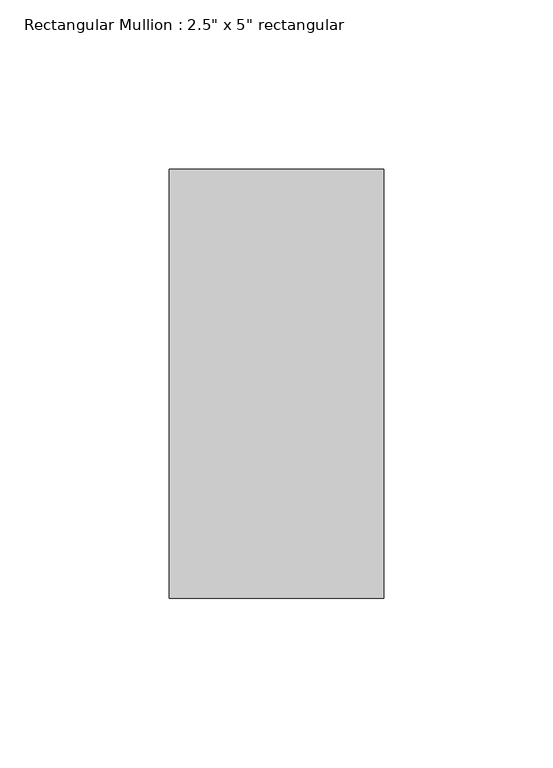
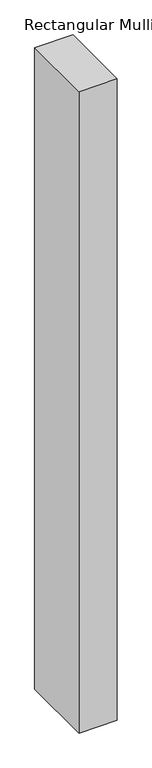
"""IFC4 building model written with IfcOpenShell, lengths in millimetres: member geometry."""

from ifc_helpers import new_model, si_unit, frame, origin, place, context, project, spatial, polyline, outline, extrude, source, transform, mapped, element, save


def member_866a01fa(model_context):
    return source(origin(), model_context, "Body", "SweptSolid", [
        extrude(outline(polyline([(31.75, 63.5), (31.75, -63.5), (-31.75, -63.5), (-31.75, 63.5), (31.75, 63.5)])), frame((0.0, 0.0, -1123.95), z_axis=(0.0, 0.0, 1.0), x_axis=(1.0, 0.0, 0.0)), (0.0, 0.0, 1.0), 1123.95),
    ])


if __name__ == "__main__":
    model = new_model("IFC4")
    model_context = context("Model", 3, world=origin())
    ifc_project = project(units=[si_unit("LENGTHUNIT", "METRE", prefix="MILLI")], contexts=[model_context])
    site = spatial("IfcSite", under=ifc_project)
    building = spatial("IfcBuilding", under=site)
    placement = place(None, origin())
    member_shape = member_866a01fa(model_context)
    element("IfcMember", 1, ObjectType="Rectangular Mullion : 2.5\" x 5\" rectangular", at=placement, inside=building, context=model_context, shape_type="MappedRepresentation", body=[
        mapped(member_shape, transform((0.0, 0.0, 0.0), x_axis=(1.0, 0.0, 0.0), y_axis=(0.0, 1.0, 0.0), z_axis=(0.0, 0.0, 1.0))),
    ])
    save(model, "model.ifc")

# Revit data of these elements
# Type "Rectangular Mullion : 2.5\" x 5\" rectangular"
#   built-in parameter 1007304 = 0.416667 (stored number, unit not read)
#   built-in parameter 1007301 = 0.104167 (stored number, unit not read)
#   built-in parameter 1007300 = 0.104167 (stored number, unit not read)
# Element 1 (IfcMember, "Rectangular Mullion : 2.5\" x 5\" rectangular")
#   Materials on its faces: "Aluminum"
# Materials
#   "Aluminum": class "Metal", colour RGB 247 247 247, transparency 0, Description = "Aluminum 6061", Cost = 0
